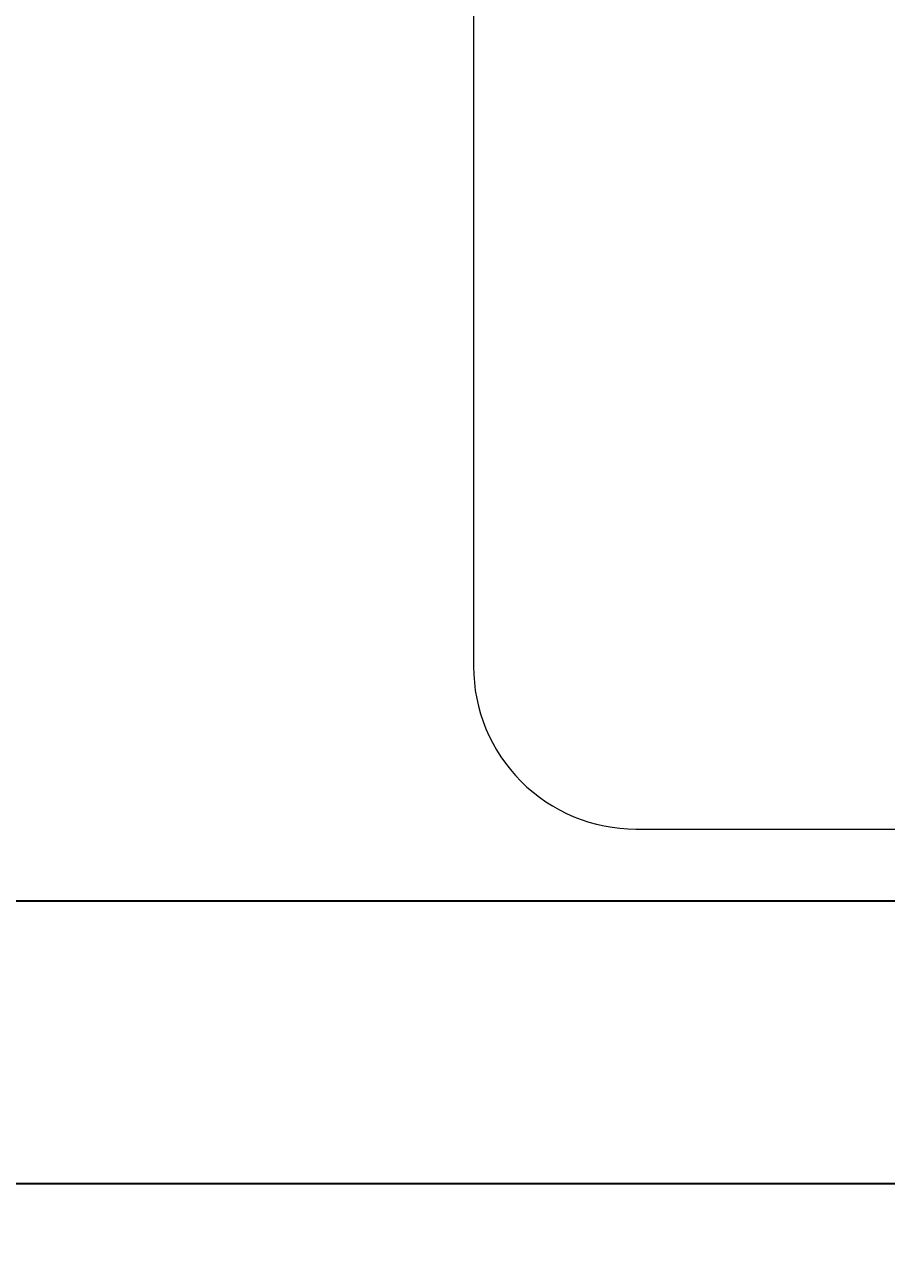
# Model space of a CAD drawing. Units: inches. Extents: x -61 to 1599, y -1316 to 257.
# Tile 33 of 204: x 91 to 109, y -790 to -763. Entities that reach past the tile are written whole.
import ezdxf

# ---------------------------------------------------------------- set-up
doc = ezdxf.new("R2010")
doc.units = ezdxf.units.IN
doc.header["$MEASUREMENT"] = 0
for name, color, linetype, lineweight in [('A-ANNO-DIMS', 2, 'Continuous', 18), ('FURNITURE', 83, 'Continuous', 18), ('WALLS', 4, 'Continuous', 35)]:
    doc.layers.add(name, color=color, linetype=linetype, lineweight=lineweight)
doc.styles.get("Standard").update_dxf_attribs({"font": 'arial.ttf'})
doc.dimstyles.get("Standard").update_dxf_attribs({"dimtxt": 0.18, "dimasz": 0.18, "dimexe": 0.18, "dimexo": 0.0625, "dimgap": 0.09, "dimtad": 0, "dimtih": 1, "dimtoh": 1, "dimdec": 0, "dimzin": 0, "dimdsep": 46, "dimlunit": 3, "dimtxsty": 'Standard', "dimcen": 0.09, "dimadec": 0, "dimazin": 0, "dimtfac": 1, "dimtdec": 0, "dimtofl": 0, "dimtmove": 0, "dimatfit": 3, "dimfxl": 1, "dimtolj": 1, "dimtzin": 0, "dimarcsym": 0})

# ---------------------------------------------------------------- blocks, each defined once
blk = doc.blocks.new('BED-DOUBLE')
blk.add_lwpolyline([(1.272, 88.537), (1.272, 3.449, 0.414214), (4.722, 0), (66.813, 0, 0.414214), (70.263, 3.449), (70.263, 88.537, 0.414214), (66.813, 91.987), (4.722, 91.987, 0.414214)], format="xyb", close=True)
blk = doc.blocks.new('*D687')
at = {"layer": 'A-ANNO-DIMS', "color": 0, "lineweight": -2, "transparency": 16777216}
for p, q in [((289.418, 181.677), (-61.077, 181.677)), ((-60.897, 181.497), (-60.897, -528.952)), ((-60.897, -1239.765), (-60.897, -529.316)), ((319.64, -1239.945), (-61.077, -1239.945))]:
    blk.add_line(p, q, dxfattribs=at)
at = {"layer": 'A-ANNO-DIMS', "color": 0, "transparency": 16777216}
for points in [[(-60.927, 181.497), (-60.867, 181.497), (-60.897, 181.677)], [(-60.927, -1239.765), (-60.867, -1239.765), (-60.897, -1239.945)]]:
    blk.add_solid(points, dxfattribs=at)
at = {"layer": 'DEFPOINTS', "color": 0, "transparency": 16777216}
for p in [(289.481, 181.677), (-60.897, -1239.945), (319.703, -1239.945)]:
    blk.add_point(p, dxfattribs=at)
at = {"layer": 'A-ANNO-DIMS', "color": 0, "transparency": 16777216, "insert": (-60.897, -529.134), "char_height": 0.18, "attachment_point": 5}
blk.add_mtext('\\A1;1421.6', dxfattribs=at)

msp = doc.modelspace()

# ---------------------------------------------------------------- linework, layer by layer
at = {"layer": 'WALLS'}
for p, q in [((14.7028, -781.9446), (237.7028, -781.9446)), ((14.7028, -787.9446), (237.7028, -787.9446))]:
    msp.add_line(p, q, dxfattribs=at)

# ---------------------------------------------------------------- block references
at = {"layer": 'FURNITURE'}
msp.add_blockref('BED-DOUBLE', (98.977, -780.4187), dxfattribs=at)

# ---------------------------------------------------------------- dimensions: what is measured, and where the dimension line sits
at = {"layer": 'A-ANNO-DIMS'}
dim = msp.add_linear_dim(base=(-60.8972, -1239.9446), p1=(289.4807, 181.6771), p2=(319.7028, -1239.9446), angle=90, dimstyle='Standard', override={"dimdec": 1, "dimlfac": 1, "dimrnd": 0, "dimzin": 0, "dimdsep": 46, "dimlunit": 2}, dxfattribs=at)
dim.commit()
dim.dimension.update_dxf_attribs({"geometry": '*D687', "text_midpoint": (-60.8972, -529.1337)})

doc.saveas('drawing.dxf')
